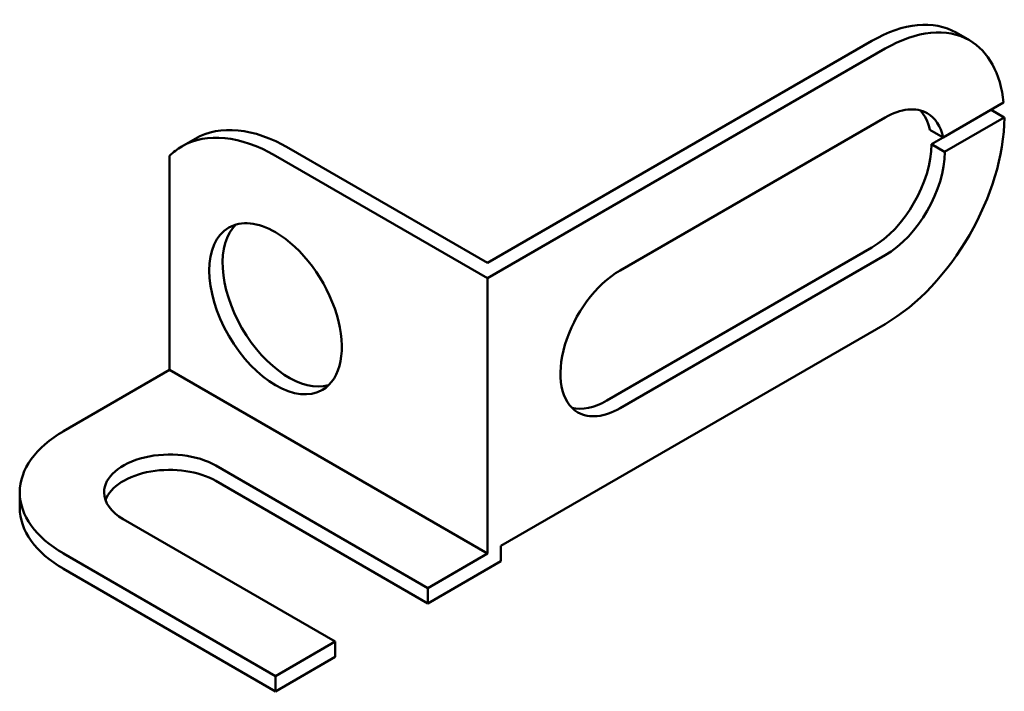
# Model space of a CAD drawing. Units: inches. Extents: x 162 to 4198, y 96 to 2472.
# Tile 1 of 1: x 4096.2 to 4198.3, y 2402.7 to 2472.4. Entities that reach past the tile are written whole.
import ezdxf

# ---------------------------------------------------------------- set-up
doc = ezdxf.new("R2010")
doc.units = ezdxf.units.IN
doc.header["$MEASUREMENT"] = 0
doc.layers.add('M-OUTL', color=7, linetype='Continuous', lineweight=50)

msp = doc.modelspace()

# ---------------------------------------------------------------- linework, layer by layer
at = {"layer": 'M-OUTL'}
for p, q in [((4193.34, 2471.01), (4194.71, 2470.22)), ((4184.59, 2470.14), (4144.72, 2447.12)), ((4185.97, 2469.35), (4144.72, 2445.54)), ((4192, 2460.13), (4198.26, 2463.75)), ((4196.96, 2463), (4198.34, 2462.21)), ((4158.47, 2446.33), (4185.97, 2462.21)), ((4192.15, 2458.63), (4198.34, 2462.21)), ((4192, 2460.13), (4190.62, 2460.93)), ((4114.38, 2459.99), (4113, 2459.2)), ((4192, 2460.13), (4190.78, 2459.43)), ((4192.15, 2458.63), (4190.78, 2459.43)), ((4111.73, 2436.01), (4111.73, 2458.24)), ((4144.72, 2445.54), (4122.72, 2458.24)), ((4124.1, 2459.03), (4144.72, 2447.12)), ((4184.59, 2448.71), (4157.09, 2432.84)), ((4158.47, 2432.04), (4185.97, 2447.92)), ((4144.72, 2445.54), (4144.72, 2416.96)), ((4146.1, 2417.76), (4185.97, 2440.77)), ((4100.73, 2429.66), (4111.73, 2436.01)), ((4144.72, 2416.96), (4111.73, 2436.01)), ((4138.53, 2413.39), (4116.54, 2426.09)), ((4138.53, 2411.8), (4116.54, 2424.5)), ((4096.17, 2421.72), (4096.17, 2423.31)), ((4128.91, 2407.83), (4106.91, 2420.53)), ((4146.1, 2416.17), (4146.1, 2417.76)), ((4122.72, 2404.26), (4100.73, 2416.96)), ((4138.53, 2413.39), (4144.72, 2416.96)), ((4122.72, 2402.67), (4100.73, 2415.37)), ((4146.1, 2416.17), (4138.53, 2411.8)), ((4138.53, 2413.39), (4138.53, 2411.8)), ((4122.72, 2404.26), (4128.91, 2407.83)), ((4128.91, 2407.83), (4128.91, 2406.25)), ((4122.72, 2402.67), (4128.91, 2406.25)), ((4122.72, 2402.67), (4122.72, 2404.26))]:
    msp.add_line(p, q, dxfattribs=at)
for centre, major_axis, start_param, end_param in [((4184.59, 2455.86), (-8.75, -15.15), 3.141593, 3.926991), ((4185.97, 2455.06), (-8.75, -15.15), 3.141593, 3.926991), ((4185.97, 2455.06), (-8.75, -15.15), 2.467536, 3.141593), ((4185.97, 2455.06), (4.37, 7.58), 0, 0.785398), ((4184.59, 2455.86), (4.37, 7.58), 5.72188, 6.125397), ((4185.97, 2455.06), (4.37, 7.58), 5.72188, 6.283185), ((4124.1, 2443.16), (9.72, -16.84), 2.356194, 3.141593), ((4185.97, 2455.06), (-8.75, -15.15), 0.785398, 2.356194), ((4122.72, 2442.36), (9.72, -16.84), 2.356194, 3.141593), ((4122.72, 2442.36), (9.72, -16.84), 3.141593, 3.28349), ((4184.59, 2455.86), (4.37, 7.58), 3.926991, 5.497787), ((4185.97, 2455.06), (4.37, 7.58), 3.926991, 5.497787), ((4124.1, 2443.16), (4.86, -8.42), 3.28349, 6.141288), ((4122.72, 2442.36), (4.86, -8.42), 2.356194, 3.141593), ((4122.72, 2442.36), (4.86, -8.42), 3.141593, 6.283185), ((4122.72, 2442.36), (4.86, -8.42), 0, 2.356194), ((4158.47, 2439.19), (4.37, 7.58), 0.785398, 3.141593), ((4157.09, 2439.98), (4.37, 7.58), 3.299381, 3.926991), ((4158.47, 2439.19), (4.37, 7.58), 3.141593, 3.926991), ((4111.73, 2423.31), (-15.55, 0), 5.497787, 6.283185), ((4111.73, 2423.31), (6.8, 0), 0.785398, 3.141593), ((4111.73, 2421.72), (6.8, 0), 0.785398, 2.938162), ((4111.73, 2423.31), (-15.55, 0), 0, 0.785398), ((4111.73, 2423.31), (6.8, 0), 3.141593, 3.926991), ((4111.73, 2421.72), (-15.55, 0), 0, 0.785398)]:
    msp.add_ellipse(centre, major_axis=major_axis, ratio=0.57735, start_param=start_param, end_param=end_param, dxfattribs=at)

doc.saveas('drawing.dxf')
